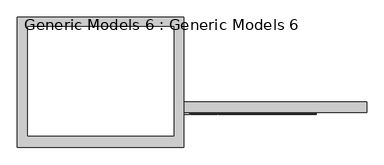
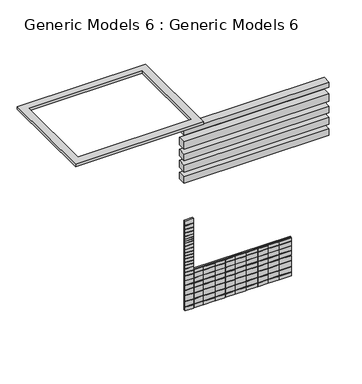
"""IFC4 building model written with IfcOpenShell, lengths in millimetres: proxy geometry, Generic Models 6 : Generic Models 6."""

from ifc_helpers import new_model, si_unit, frame, origin, place, context, project, spatial, polyline, outline, extrude, faceted_brep, source, transform, mapped, element, save


def generic_models_6_generic_models_6_0c77f430(model_context):
    return source(origin(), model_context, "Body", "SolidModel", [
        extrude(outline(polyline([(-18013.9734486, -8229.0592534), (-14420.7831929, -8229.0592534), (-14420.7831929, -11048.4592534), (-18013.9734486, -11048.4592534), (-18013.9734486, -8229.0592534)]), holes=[polyline([(-17794.9964661, -10800.2393368), (-14630.8767684, -10800.2393368), (-14630.8767684, -8432.2592534), (-17794.9964661, -8432.2592534), (-17794.9964661, -10800.2393368)])]), frame((0.0, 0.0, 8571.3431053), z_axis=(0.0, 0.0, 1.0), x_axis=(1.0, 0.0, 0.0)), (0.0, 0.0, 1.0), 76.2),
        extrude(outline(polyline([(-14524.7437117, -10286.4592534), (-14524.7437117, -10057.8592534), (-10464.7331929, -10057.8592534), (-10464.7331929, -10286.4592534), (-14524.7437117, -10286.4592534)])), frame((0.0, 0.0, 6400.8), z_axis=(0.0, 0.0, 1.0), x_axis=(1.0, 0.0, 0.0)), (0.0, 0.0, 1.0), 191.3675565),
        extrude(outline(polyline([(-14524.7437117, -10286.4592534), (-14524.7437117, -10057.8592534), (-10464.7331929, -10057.8592534), (-10464.7331929, -10286.4592534), (-14524.7437117, -10286.4592534)])), frame((0.0, 0.0, 6738.1730597), z_axis=(0.0, 0.0, 1.0), x_axis=(1.0, 0.0, 0.0)), (0.0, 0.0, 1.0), 204.0095282),
        extrude(outline(polyline([(-14524.7437117, -10286.4592534), (-14524.7437117, -10057.8592534), (-10464.7331929, -10057.8592534), (-10464.7331929, -10286.4592534), (-14524.7437117, -10286.4592534)])), frame((0.0, 0.0, 7077.9317925), z_axis=(0.0, 0.0, 1.0), x_axis=(1.0, 0.0, 0.0)), (0.0, 0.0, 1.0), 192.5683417),
        extrude(outline(polyline([(-14524.7437117, -10286.4592534), (-14524.7437117, -10057.8592534), (-10464.7331929, -10057.8592534), (-10464.7331929, -10286.4592534), (-14524.7437117, -10286.4592534)])), frame((0.0, 0.0, 7413.8898365), z_axis=(0.0, 0.0, 1.0), x_axis=(1.0, 0.0, 0.0)), (0.0, 0.0, 1.0), 213.9956527),
        extrude(outline(polyline([(-14524.7437117, -10286.4592534), (-14524.7437117, -10057.8592534), (-10464.7331929, -10057.8592534), (-10464.7331929, -10286.4592534), (-14524.7437117, -10286.4592534)])), frame((0.0, 0.0, 7820.9092835), z_axis=(0.0, 0.0, 1.0), x_axis=(1.0, 0.0, 0.0)), (0.0, 0.0, 1.0), 157.6710883),
        faceted_brep([(-14293.7831929, -10337.2592534, 5313.3697962), (-14524.7437117, -10337.2592534, 5313.3697962), (-14524.7437117, -10337.2592534, 5188.1331788), (-14293.7831929, -10337.2592534, 5188.1331788), (-11550.5831929, -10337.2592534, 3695.8817592), (-11550.5831929, -10337.2592534, 3780.6568837), (-11880.9442119, -10337.2592534, 3780.6568837), (-11880.9442119, -10337.2592534, 3695.8817592), (-11550.5831929, -10337.2592534, 3547.0366558), (-11550.5831929, -10337.2592534, 3680.189393), (-11880.9442119, -10337.2592534, 3680.189393), (-11880.9442119, -10337.2592534, 3547.0366558), (-11550.5831929, -10337.2592534, 3417.1914801), (-11550.5831929, -10337.2592534, 3542.5886948), (-11880.9442119, -10337.2592534, 3542.5886948), (-11880.9442119, -10337.2592534, 3417.1914801), (-11550.5831929, -10337.2592534, 3270.1734591), (-11550.5831929, -10337.2592534, 3393.2583138), (-11880.9442119, -10337.2592534, 3393.2583138), (-11880.9442119, -10337.2592534, 3270.1734591), (-11550.5831929, -10337.2592534, 3111.840506), (-11550.5831929, -10337.2592534, 3253.9449104), (-11880.9442119, -10337.2592534, 3253.9449104), (-11880.9442119, -10337.2592534, 3111.840506), (-11550.5831929, -10337.2592534, 2938.7596873), (-11550.5831929, -10337.2592534, 3096.8139071), (-11880.9442119, -10337.2592534, 3096.8139071), (-11880.9442119, -10337.2592534, 2938.7596873), (-11550.5831929, -10337.2592534, 2659.3923672), (-11550.5831929, -10337.2592534, 2760.4299366), (-11880.9442119, -10337.2592534, 2760.4299366), (-11880.9442119, -10337.2592534, 2659.3923672), (-11550.5831929, -10337.2592534, 2780.6285186), (-11550.5831929, -10337.2592534, 2920.5978973), (-11880.9442119, -10337.2592534, 2920.5978973), (-11880.9442119, -10337.2592534, 2780.6285186), (-14293.7831929, -10337.2592534, 5069.4562317), (-14293.7831929, -10337.2592534, 5168.2265161), (-14524.7437117, -10337.2592534, 5168.2265161), (-14524.7437117, -10337.2592534, 5069.4562317), (-14293.7831929, -10337.2592534, 4965.1249586), (-14293.7831929, -10337.2592534, 5057.6988625), (-14524.7437117, -10337.2592534, 5057.6988625), (-14524.7437117, -10337.2592534, 4965.1249586), (-14293.7831929, -10337.2592534, 4865.3991355), (-14293.7831929, -10337.2592534, 4953.6426938), (-14524.7437117, -10337.2592534, 4953.6426938), (-14524.7437117, -10337.2592534, 4865.3991355), (-14293.7831929, -10337.2592534, 4781.0487347), (-14293.7831929, -10337.2592534, 4856.4332696), (-14524.7437117, -10337.2592534, 4856.4332696), (-14524.7437117, -10337.2592534, 4781.0487347), (-14293.7831929, -10337.2592534, 4721.3683685), (-14293.7831929, -10337.2592534, 4774.4107583), (-14524.7437117, -10337.2592534, 4774.4107583), (-14524.7437117, -10337.2592534, 4721.3683685), (-14293.7831929, -10337.2592534, 4665.5616831), (-14293.7831929, -10337.2592534, 4715.3945526), (-14524.7437117, -10337.2592534, 4715.3945526), (-14524.7437117, -10337.2592534, 4665.5616831), (-14293.7831929, -10337.2592534, 4571.464179), (-14293.7831929, -10337.2592534, 4658.9302933), (-14524.7437117, -10337.2592534, 4658.9302933), (-14524.7437117, -10337.2592534, 4571.464179), (-14293.7831929, -10337.2592534, 4470.4894096), (-14293.7831929, -10337.2592534, 4556.4765983), (-14524.7437117, -10337.2592534, 4556.4765983), (-14524.7437117, -10337.2592534, 4470.4894096), (-14293.7831929, -10337.2592534, 4373.4391753), (-14293.7831929, -10337.2592534, 4459.0931873), (-14524.7437117, -10337.2592534, 4459.0931873), (-14524.7437117, -10337.2592534, 4373.4391753), (-14293.7831929, -10337.2592534, 4282.1802011), (-14293.7831929, -10337.2592534, 4359.300461), (-14524.7437117, -10337.2592534, 4359.300461), (-14524.7437117, -10337.2592534, 4282.1802011), (-14293.7831929, -10337.2592534, 4193.4919021), (-14293.7831929, -10337.2592534, 4269.3268244), (-14524.7437117, -10337.2592534, 4269.3268244), (-14524.7437117, -10337.2592534, 4193.4919021), (-14293.7831929, -10337.2592534, 4094.064607), (-14293.7831929, -10337.2592534, 4178.0678501), (-14524.7437117, -10337.2592534, 4178.0678501), (-14524.7437117, -10337.2592534, 4094.064607), (-14293.7831929, -10337.2592534, 4000.5723585), (-14293.7831929, -10337.2592534, 4078.7658754), (-14524.7437117, -10337.2592534, 4078.7658754), (-14524.7437117, -10337.2592534, 4000.5723585), (-14293.7831929, -10337.2592534, 3799.5834003), (-14293.7831929, -10337.2592534, 3891.5162081), (-14524.7437117, -10337.2592534, 3891.5162081), (-14524.7437117, -10337.2592534, 3799.5834003), (-14293.7831929, -10337.2592534, 3900.2806738), (-14293.7831929, -10337.2592534, 3986.3810817), (-14524.7437117, -10337.2592534, 3986.3810817), (-14524.7437117, -10337.2592534, 3900.2806738), (-14524.7437117, -10337.2592534, 3780.6568837), (-14524.7437117, -10337.2592534, 3695.8817592), (-14293.7831929, -10337.2592534, 3695.8817592), (-14293.7831929, -10337.2592534, 3780.6568837), (-14524.7437117, -10337.2592534, 3680.189393), (-14524.7437117, -10337.2592534, 3547.0366558), (-14293.7831929, -10337.2592534, 3547.0366558), (-14293.7831929, -10337.2592534, 3680.189393), (-14524.7437117, -10337.2592534, 3542.5886948), (-14524.7437117, -10337.2592534, 3417.1914801), (-14293.7831929, -10337.2592534, 3417.1914801), (-14293.7831929, -10337.2592534, 3542.5886948), (-14524.7437117, -10337.2592534, 3393.2583138), (-14524.7437117, -10337.2592534, 3270.1734591), (-14293.7831929, -10337.2592534, 3270.1734591), (-14293.7831929, -10337.2592534, 3393.2583138), (-14524.7437117, -10337.2592534, 3253.9449104), (-14524.7437117, -10337.2592534, 3111.840506), (-14293.7831929, -10337.2592534, 3111.840506), (-14293.7831929, -10337.2592534, 3253.9449104), (-14524.7437117, -10337.2592534, 3096.8139071), (-14524.7437117, -10337.2592534, 2938.7596873), (-14293.7831929, -10337.2592534, 2938.7596873), (-14293.7831929, -10337.2592534, 3096.8139071), (-14524.7437117, -10337.2592534, 2760.4299366), (-14524.7437117, -10337.2592534, 2659.3923672), (-14293.7831929, -10337.2592534, 2659.3923672), (-14293.7831929, -10337.2592534, 2760.4299366), (-14524.7437117, -10337.2592534, 2920.5978973), (-14524.7437117, -10337.2592534, 2780.6285186), (-14293.7831929, -10337.2592534, 2780.6285186), (-14293.7831929, -10337.2592534, 2920.5978973), (-14277.8960614, -10337.2592534, 2659.3923672), (-14019.6359859, -10337.2592534, 2659.3923672), (-14019.6359859, -10337.2592534, 2760.4299366), (-14277.8960614, -10337.2592534, 2760.4299366), (-14004.4843067, -10337.2592534, 2659.3923672), (-13695.1641924, -10337.2592534, 2659.3923672), (-13695.1641924, -10337.2592534, 2760.4299366), (-14004.4843067, -10337.2592534, 2760.4299366), (-13674.725498, -10337.2592534, 2659.3923672), (-13411.1331929, -10337.2592534, 2659.3923672), (-13411.1331929, -10337.2592534, 2760.4299366), (-13674.725498, -10337.2592534, 2760.4299366), (-13398.4331929, -10337.2592534, 2659.3923672), (-13132.6036786, -10337.2592534, 2659.3923672), (-13132.6036786, -10337.2592534, 2760.4299366), (-13398.4331929, -10337.2592534, 2760.4299366), (-13122.8488627, -10337.2592534, 2659.3923672), (-12816.2756326, -10337.2592534, 2659.3923672), (-12816.2756326, -10337.2592534, 2760.4299366), (-13122.8488627, -10337.2592534, 2760.4299366), (-12805.7258669, -10337.2592534, 2659.3923672), (-12496.7331929, -10337.2592534, 2659.3923672), (-12496.7331929, -10337.2592534, 2760.4299366), (-12805.7258669, -10337.2592534, 2760.4299366), (-12491.0846074, -10337.2592534, 2659.3923672), (-12209.2160936, -10337.2592534, 2659.3923672), (-12209.2160936, -10337.2592534, 2760.4299366), (-12491.0846074, -10337.2592534, 2760.4299366), (-12202.6421379, -10337.2592534, 2659.3923672), (-11888.3927856, -10337.2592534, 2659.3923672), (-11888.3927856, -10337.2592534, 2760.4299366), (-12202.6421379, -10337.2592534, 2760.4299366), (-14019.6359859, -10337.2592534, 3780.6568837), (-14277.8960614, -10337.2592534, 3780.6568837), (-14277.8960614, -10337.2592534, 3695.8817592), (-14019.6359859, -10337.2592534, 3695.8817592), (-13695.1641924, -10337.2592534, 3780.6568837), (-14004.4843067, -10337.2592534, 3780.6568837), (-14004.4843067, -10337.2592534, 3695.8817592), (-13695.1641924, -10337.2592534, 3695.8817592), (-13411.1331929, -10337.2592534, 3780.6568837), (-13674.725498, -10337.2592534, 3780.6568837), (-13674.725498, -10337.2592534, 3695.8817592), (-13411.1331929, -10337.2592534, 3695.8817592), (-13132.6036786, -10337.2592534, 3780.6568837), (-13398.4331929, -10337.2592534, 3780.6568837), (-13398.4331929, -10337.2592534, 3695.8817592), (-13132.6036786, -10337.2592534, 3695.8817592), (-12816.2756326, -10337.2592534, 3780.6568837), (-13122.8488627, -10337.2592534, 3780.6568837), (-13122.8488627, -10337.2592534, 3695.8817592), (-12816.2756326, -10337.2592534, 3695.8817592), (-12496.7331929, -10337.2592534, 3780.6568837), (-12805.7258669, -10337.2592534, 3780.6568837), (-12805.7258669, -10337.2592534, 3695.8817592), (-12496.7331929, -10337.2592534, 3695.8817592), (-12209.2160936, -10337.2592534, 3780.6568837), (-12491.0846074, -10337.2592534, 3780.6568837), (-12491.0846074, -10337.2592534, 3695.8817592), (-12209.2160936, -10337.2592534, 3695.8817592), (-11888.3927856, -10337.2592534, 3780.6568837), (-12202.6421379, -10337.2592534, 3780.6568837), (-12202.6421379, -10337.2592534, 3695.8817592), (-11888.3927856, -10337.2592534, 3695.8817592), (-14019.6359859, -10337.2592534, 3680.189393), (-14277.8960614, -10337.2592534, 3680.189393), (-14277.8960614, -10337.2592534, 3547.0366558), (-14019.6359859, -10337.2592534, 3547.0366558), (-13695.1641924, -10337.2592534, 3680.189393), (-14004.4843067, -10337.2592534, 3680.189393), (-14004.4843067, -10337.2592534, 3547.0366558), (-13695.1641924, -10337.2592534, 3547.0366558), (-13411.1331929, -10337.2592534, 3680.189393), (-13674.725498, -10337.2592534, 3680.189393), (-13674.725498, -10337.2592534, 3547.0366558), (-13411.1331929, -10337.2592534, 3547.0366558), (-13132.6036786, -10337.2592534, 3680.189393), (-13398.4331929, -10337.2592534, 3680.189393), (-13398.4331929, -10337.2592534, 3547.0366558), (-13132.6036786, -10337.2592534, 3547.0366558), (-12816.2756326, -10337.2592534, 3680.189393), (-13122.8488627, -10337.2592534, 3680.189393), (-13122.8488627, -10337.2592534, 3547.0366558), (-12816.2756326, -10337.2592534, 3547.0366558), (-12496.7331929, -10337.2592534, 3680.189393), (-12805.7258669, -10337.2592534, 3680.189393), (-12805.7258669, -10337.2592534, 3547.0366558), (-12496.7331929, -10337.2592534, 3547.0366558), (-12209.2160936, -10337.2592534, 3680.189393), (-12491.0846074, -10337.2592534, 3680.189393), (-12491.0846074, -10337.2592534, 3547.0366558), (-12209.2160936, -10337.2592534, 3547.0366558), (-11888.3927856, -10337.2592534, 3680.189393), (-12202.6421379, -10337.2592534, 3680.189393), (-12202.6421379, -10337.2592534, 3547.0366558), (-11888.3927856, -10337.2592534, 3547.0366558), (-14019.6359859, -10337.2592534, 3542.5886948), (-14277.8960614, -10337.2592534, 3542.5886948), (-14277.8960614, -10337.2592534, 3417.1914801), (-14019.6359859, -10337.2592534, 3417.1914801), (-13695.1641924, -10337.2592534, 3542.5886948), (-14004.4843067, -10337.2592534, 3542.5886948), (-14004.4843067, -10337.2592534, 3417.1914801), (-13695.1641924, -10337.2592534, 3417.1914801), (-13411.1331929, -10337.2592534, 3542.5886948), (-13674.725498, -10337.2592534, 3542.5886948), (-13674.725498, -10337.2592534, 3417.1914801), (-13411.1331929, -10337.2592534, 3417.1914801), (-13132.6036786, -10337.2592534, 3542.5886948), (-13398.4331929, -10337.2592534, 3542.5886948), (-13398.4331929, -10337.2592534, 3417.1914801), (-13132.6036786, -10337.2592534, 3417.1914801), (-12816.2756326, -10337.2592534, 3542.5886948), (-13122.8488627, -10337.2592534, 3542.5886948), (-13122.8488627, -10337.2592534, 3417.1914801), (-12816.2756326, -10337.2592534, 3417.1914801), (-12496.7331929, -10337.2592534, 3542.5886948), (-12805.7258669, -10337.2592534, 3542.5886948), (-12805.7258669, -10337.2592534, 3417.1914801), (-12496.7331929, -10337.2592534, 3417.1914801), (-12209.2160936, -10337.2592534, 3542.5886948), (-12491.0846074, -10337.2592534, 3542.5886948), (-12491.0846074, -10337.2592534, 3417.1914801), (-12209.2160936, -10337.2592534, 3417.1914801), (-11888.3927856, -10337.2592534, 3542.5886948), (-12202.6421379, -10337.2592534, 3542.5886948), (-12202.6421379, -10337.2592534, 3417.1914801), (-11888.3927856, -10337.2592534, 3417.1914801), (-14019.6359859, -10337.2592534, 3393.2583138), (-14277.8960614, -10337.2592534, 3393.2583138), (-14277.8960614, -10337.2592534, 3270.1734591), (-14019.6359859, -10337.2592534, 3270.1734591), (-13695.1641924, -10337.2592534, 3393.2583138), (-14004.4843067, -10337.2592534, 3393.2583138), (-14004.4843067, -10337.2592534, 3270.1734591), (-13695.1641924, -10337.2592534, 3270.1734591), (-13411.1331929, -10337.2592534, 3393.2583138), (-13674.725498, -10337.2592534, 3393.2583138), (-13674.725498, -10337.2592534, 3270.1734591), (-13411.1331929, -10337.2592534, 3270.1734591), (-13132.6036786, -10337.2592534, 3393.2583138), (-13398.4331929, -10337.2592534, 3393.2583138), (-13398.4331929, -10337.2592534, 3270.1734591), (-13132.6036786, -10337.2592534, 3270.1734591), (-12816.2756326, -10337.2592534, 3393.2583138), (-13122.8488627, -10337.2592534, 3393.2583138), (-13122.8488627, -10337.2592534, 3270.1734591), (-12816.2756326, -10337.2592534, 3270.1734591), (-12496.7331929, -10337.2592534, 3393.2583138), (-12805.7258669, -10337.2592534, 3393.2583138), (-12805.7258669, -10337.2592534, 3270.1734591), (-12496.7331929, -10337.2592534, 3270.1734591), (-12209.2160936, -10337.2592534, 3393.2583138), (-12491.0846074, -10337.2592534, 3393.2583138), (-12491.0846074, -10337.2592534, 3270.1734591), (-12209.2160936, -10337.2592534, 3270.1734591), (-11888.3927856, -10337.2592534, 3393.2583138), (-12202.6421379, -10337.2592534, 3393.2583138), (-12202.6421379, -10337.2592534, 3270.1734591), (-11888.3927856, -10337.2592534, 3270.1734591), (-14019.6359859, -10337.2592534, 3253.9449104), (-14277.8960614, -10337.2592534, 3253.9449104), (-14277.8960614, -10337.2592534, 3111.840506), (-14019.6359859, -10337.2592534, 3111.840506), (-13695.1641924, -10337.2592534, 3253.9449104), (-14004.4843067, -10337.2592534, 3253.9449104), (-14004.4843067, -10337.2592534, 3111.840506), (-13695.1641924, -10337.2592534, 3111.840506), (-13411.1331929, -10337.2592534, 3253.9449104), (-13674.725498, -10337.2592534, 3253.9449104), (-13674.725498, -10337.2592534, 3111.840506), (-13411.1331929, -10337.2592534, 3111.840506), (-13132.6036786, -10337.2592534, 3253.9449104), (-13398.4331929, -10337.2592534, 3253.9449104), (-13398.4331929, -10337.2592534, 3111.840506), (-13132.6036786, -10337.2592534, 3111.840506), (-12816.2756326, -10337.2592534, 3253.9449104), (-13122.8488627, -10337.2592534, 3253.9449104), (-13122.8488627, -10337.2592534, 3111.840506), (-12816.2756326, -10337.2592534, 3111.840506), (-12496.7331929, -10337.2592534, 3253.9449104), (-12805.7258669, -10337.2592534, 3253.9449104), (-12805.7258669, -10337.2592534, 3111.840506), (-12496.7331929, -10337.2592534, 3111.840506), (-12209.2160936, -10337.2592534, 3253.9449104), (-12491.0846074, -10337.2592534, 3253.9449104), (-12491.0846074, -10337.2592534, 3111.840506), (-12209.2160936, -10337.2592534, 3111.840506), (-11888.3927856, -10337.2592534, 3253.9449104), (-12202.6421379, -10337.2592534, 3253.9449104), (-12202.6421379, -10337.2592534, 3111.840506), (-11888.3927856, -10337.2592534, 3111.840506), (-14019.6359859, -10337.2592534, 3096.8139071), (-14277.8960614, -10337.2592534, 3096.8139071), (-14277.8960614, -10337.2592534, 2938.7596873), (-14019.6359859, -10337.2592534, 2938.7596873), (-13695.1641924, -10337.2592534, 3096.8139071), (-14004.4843067, -10337.2592534, 3096.8139071), (-14004.4843067, -10337.2592534, 2938.7596873), (-13695.1641924, -10337.2592534, 2938.7596873), (-13411.1331929, -10337.2592534, 3096.8139071), (-13674.725498, -10337.2592534, 3096.8139071), (-13674.725498, -10337.2592534, 2938.7596873), (-13411.1331929, -10337.2592534, 2938.7596873), (-13132.6036786, -10337.2592534, 3096.8139071), (-13398.4331929, -10337.2592534, 3096.8139071), (-13398.4331929, -10337.2592534, 2938.7596873), (-13132.6036786, -10337.2592534, 2938.7596873), (-12816.2756326, -10337.2592534, 3096.8139071), (-13122.8488627, -10337.2592534, 3096.8139071), (-13122.8488627, -10337.2592534, 2938.7596873), (-12816.2756326, -10337.2592534, 2938.7596873), (-12496.7331929, -10337.2592534, 3096.8139071), (-12805.7258669, -10337.2592534, 3096.8139071), (-12805.7258669, -10337.2592534, 2938.7596873), (-12496.7331929, -10337.2592534, 2938.7596873), (-12209.2160936, -10337.2592534, 3096.8139071), (-12491.0846074, -10337.2592534, 3096.8139071), (-12491.0846074, -10337.2592534, 2938.7596873), (-12209.2160936, -10337.2592534, 2938.7596873), (-11888.3927856, -10337.2592534, 3096.8139071), (-12202.6421379, -10337.2592534, 3096.8139071), (-12202.6421379, -10337.2592534, 2938.7596873), (-11888.3927856, -10337.2592534, 2938.7596873), (-14019.6359859, -10337.2592534, 2920.5978973), (-14277.8960614, -10337.2592534, 2920.5978973), (-14277.8960614, -10337.2592534, 2780.6285186), (-14019.6359859, -10337.2592534, 2780.6285186), (-13695.1641924, -10337.2592534, 2920.5978973), (-14004.4843067, -10337.2592534, 2920.5978973), (-14004.4843067, -10337.2592534, 2780.6285186), (-13695.1641924, -10337.2592534, 2780.6285186), (-13411.1331929, -10337.2592534, 2920.5978973), (-13674.725498, -10337.2592534, 2920.5978973), (-13674.725498, -10337.2592534, 2780.6285186), (-13411.1331929, -10337.2592534, 2780.6285186), (-13132.6036786, -10337.2592534, 2920.5978973), (-13398.4331929, -10337.2592534, 2920.5978973), (-13398.4331929, -10337.2592534, 2780.6285186), (-13132.6036786, -10337.2592534, 2780.6285186), (-12816.2756326, -10337.2592534, 2920.5978973), (-13122.8488627, -10337.2592534, 2920.5978973), (-13122.8488627, -10337.2592534, 2780.6285186), (-12816.2756326, -10337.2592534, 2780.6285186), (-12496.7331929, -10337.2592534, 2920.5978973), (-12805.7258669, -10337.2592534, 2920.5978973), (-12805.7258669, -10337.2592534, 2780.6285186), (-12496.7331929, -10337.2592534, 2780.6285186), (-12209.2160936, -10337.2592534, 2920.5978973), (-12491.0846074, -10337.2592534, 2920.5978973), (-12491.0846074, -10337.2592534, 2780.6285186), (-12209.2160936, -10337.2592534, 2780.6285186), (-11888.3927856, -10337.2592534, 2920.5978973), (-12202.6421379, -10337.2592534, 2920.5978973), (-12202.6421379, -10337.2592534, 2780.6285186), (-11888.3927856, -10337.2592534, 2780.6285186), (-11550.5831929, -10286.4592534, 3799.5834003), (-11550.5831929, -10286.4592534, 2659.3923672), (-14524.7437117, -10286.4592534, 2659.3923672), (-14524.7437117, -10286.4592534, 5313.3697962), (-14293.7831929, -10286.4592534, 5313.3697962), (-14293.7831929, -10286.4592534, 3799.5834003), (-14293.7831929, -10311.8592534, 3799.5834003), (-11550.5831929, -10311.8592534, 3799.5834003), (-14524.7437117, -10311.8592534, 2760.4299366), (-14524.7437117, -10311.8592534, 2780.6285186), (-14524.7437117, -10311.8592534, 2920.5978973), (-14524.7437117, -10311.8592534, 2938.7596873), (-14524.7437117, -10311.8592534, 3096.8139071), (-14524.7437117, -10311.8592534, 3111.840506), (-14524.7437117, -10311.8592534, 3253.9449104), (-14524.7437117, -10311.8592534, 3270.1734591), (-14524.7437117, -10311.8592534, 3393.2583138), (-14524.7437117, -10311.8592534, 3417.1914801), (-14524.7437117, -10311.8592534, 3542.5886948), (-14524.7437117, -10311.8592534, 3547.0366558), (-14524.7437117, -10311.8592534, 3680.189393), (-14524.7437117, -10311.8592534, 3695.8817592), (-14524.7437117, -10311.8592534, 3780.6568837), (-14524.7437117, -10311.8592534, 3799.5834003), (-14524.7437117, -10311.8592534, 3891.5162081), (-14524.7437117, -10311.8592534, 3900.2806738), (-14524.7437117, -10311.8592534, 3986.3810817), (-14524.7437117, -10311.8592534, 4000.5723585), (-14524.7437117, -10311.8592534, 4078.7658754), (-14524.7437117, -10311.8592534, 4094.064607), (-14524.7437117, -10311.8592534, 4178.0678501), (-14524.7437117, -10311.8592534, 4193.4919021), (-14524.7437117, -10311.8592534, 4269.3268244), (-14524.7437117, -10311.8592534, 4282.1802011), (-14524.7437117, -10311.8592534, 4359.300461), (-14524.7437117, -10311.8592534, 4373.4391753), (-14524.7437117, -10311.8592534, 4459.0931873), (-14524.7437117, -10311.8592534, 4470.4894096), (-14524.7437117, -10311.8592534, 4556.4765983), (-14524.7437117, -10311.8592534, 4571.464179), (-14524.7437117, -10311.8592534, 4658.9302933), (-14524.7437117, -10311.8592534, 4665.5616831), (-14524.7437117, -10311.8592534, 4715.3945526), (-14524.7437117, -10311.8592534, 4721.3683685), (-14524.7437117, -10311.8592534, 4774.4107583), (-14524.7437117, -10311.8592534, 4781.0487347), (-14524.7437117, -10311.8592534, 4856.4332696), (-14524.7437117, -10311.8592534, 4865.3991355), (-14524.7437117, -10311.8592534, 4953.6426938), (-14524.7437117, -10311.8592534, 4965.1249586), (-14524.7437117, -10311.8592534, 5057.6988625), (-14524.7437117, -10311.8592534, 5069.4562317), (-14524.7437117, -10311.8592534, 5168.2265161), (-14524.7437117, -10311.8592534, 5188.1331788), (-11880.9442119, -10311.8592534, 2659.3923672), (-11888.3927856, -10311.8592534, 2659.3923672), (-12202.6421379, -10311.8592534, 2659.3923672), (-12209.2160936, -10311.8592534, 2659.3923672), (-12491.0846074, -10311.8592534, 2659.3923672), (-12496.7331929, -10311.8592534, 2659.3923672), (-12805.7258669, -10311.8592534, 2659.3923672), (-12816.2756326, -10311.8592534, 2659.3923672), (-13122.8488627, -10311.8592534, 2659.3923672), (-13132.6036786, -10311.8592534, 2659.3923672), (-13398.4331929, -10311.8592534, 2659.3923672), (-13411.1331929, -10311.8592534, 2659.3923672), (-13674.725498, -10311.8592534, 2659.3923672), (-13695.1641924, -10311.8592534, 2659.3923672), (-14004.4843067, -10311.8592534, 2659.3923672), (-14019.6359859, -10311.8592534, 2659.3923672), (-14277.8960614, -10311.8592534, 2659.3923672), (-14293.7831929, -10311.8592534, 2659.3923672), (-11550.5831929, -10311.8592534, 3780.6568837), (-11550.5831929, -10311.8592534, 3695.8817592), (-11550.5831929, -10311.8592534, 3680.189393), (-11550.5831929, -10311.8592534, 3547.0366558), (-11550.5831929, -10311.8592534, 3542.5886948), (-11550.5831929, -10311.8592534, 3417.1914801), (-11550.5831929, -10311.8592534, 3393.2583138), (-11550.5831929, -10311.8592534, 3270.1734591), (-11550.5831929, -10311.8592534, 3253.9449104), (-11550.5831929, -10311.8592534, 3111.840506), (-11550.5831929, -10311.8592534, 3096.8139071), (-11550.5831929, -10311.8592534, 2938.7596873), (-11550.5831929, -10311.8592534, 2920.5978973), (-11550.5831929, -10311.8592534, 2780.6285186), (-11550.5831929, -10311.8592534, 2760.4299366), (-14293.7831929, -10311.8592534, 5188.1331788), (-14293.7831929, -10311.8592534, 5168.2265161), (-14293.7831929, -10311.8592534, 5069.4562317), (-14293.7831929, -10311.8592534, 5057.6988625), (-14293.7831929, -10311.8592534, 4965.1249586), (-14293.7831929, -10311.8592534, 4953.6426938), (-14293.7831929, -10311.8592534, 4865.3991355), (-14293.7831929, -10311.8592534, 4856.4332696), (-14293.7831929, -10311.8592534, 4781.0487347), (-14293.7831929, -10311.8592534, 4774.4107583), (-14293.7831929, -10311.8592534, 4721.3683685), (-14293.7831929, -10311.8592534, 4715.3945526), (-14293.7831929, -10311.8592534, 4665.5616831), (-14293.7831929, -10311.8592534, 4658.9302933), (-14293.7831929, -10311.8592534, 4571.464179), (-14293.7831929, -10311.8592534, 4556.4765983), (-14293.7831929, -10311.8592534, 4470.4894096), (-14293.7831929, -10311.8592534, 4459.0931873), (-14293.7831929, -10311.8592534, 4373.4391753), (-14293.7831929, -10311.8592534, 4359.300461), (-14293.7831929, -10311.8592534, 4282.1802011), (-14293.7831929, -10311.8592534, 4269.3268244), (-14293.7831929, -10311.8592534, 4193.4919021), (-14293.7831929, -10311.8592534, 4178.0678501), (-14293.7831929, -10311.8592534, 4094.064607), (-14293.7831929, -10311.8592534, 4078.7658754), (-14293.7831929, -10311.8592534, 4000.5723585), (-14293.7831929, -10311.8592534, 3986.3810817), (-14293.7831929, -10311.8592534, 3900.2806738), (-14293.7831929, -10311.8592534, 3891.5162081), (-14293.7831929, -10311.8592534, 3780.6568837), (-14293.7831929, -10311.8592534, 3695.8817592), (-14293.7831929, -10311.8592534, 3680.189393), (-14293.7831929, -10311.8592534, 3547.0366558), (-14293.7831929, -10311.8592534, 3542.5886948), (-14293.7831929, -10311.8592534, 3417.1914801), (-14293.7831929, -10311.8592534, 3393.2583138), (-14293.7831929, -10311.8592534, 3270.1734591), (-14293.7831929, -10311.8592534, 3253.9449104), (-14293.7831929, -10311.8592534, 3111.840506), (-14293.7831929, -10311.8592534, 3096.8139071), (-14293.7831929, -10311.8592534, 2938.7596873), (-14293.7831929, -10311.8592534, 2920.5978973), (-14293.7831929, -10311.8592534, 2780.6285186), (-14293.7831929, -10311.8592534, 2760.4299366), (-14277.8960614, -10311.8592534, 2760.4299366), (-14019.6359859, -10311.8592534, 2760.4299366), (-14004.4843067, -10311.8592534, 2760.4299366), (-13695.1641924, -10311.8592534, 2760.4299366), (-13674.725498, -10311.8592534, 2760.4299366), (-13411.1331929, -10311.8592534, 2760.4299366), (-13398.4331929, -10311.8592534, 2760.4299366), (-13132.6036786, -10311.8592534, 2760.4299366), (-13122.8488627, -10311.8592534, 2760.4299366), (-12816.2756326, -10311.8592534, 2760.4299366), (-12805.7258669, -10311.8592534, 2760.4299366), (-12496.7331929, -10311.8592534, 2760.4299366), (-12491.0846074, -10311.8592534, 2760.4299366), (-12209.2160936, -10311.8592534, 2760.4299366), (-12202.6421379, -10311.8592534, 2760.4299366), (-11888.3927856, -10311.8592534, 2760.4299366), (-11880.9442119, -10311.8592534, 2760.4299366), (-11880.9442119, -10311.8592534, 2780.6285186), (-11880.9442119, -10311.8592534, 2920.5978973), (-11880.9442119, -10311.8592534, 2938.7596873), (-11880.9442119, -10311.8592534, 3096.8139071), (-11880.9442119, -10311.8592534, 3111.840506), (-11880.9442119, -10311.8592534, 3253.9449104), (-11880.9442119, -10311.8592534, 3270.1734591), (-11880.9442119, -10311.8592534, 3393.2583138), (-11880.9442119, -10311.8592534, 3417.1914801), (-11880.9442119, -10311.8592534, 3542.5886948), (-11880.9442119, -10311.8592534, 3547.0366558), (-11880.9442119, -10311.8592534, 3680.189393), (-11880.9442119, -10311.8592534, 3695.8817592), (-11880.9442119, -10311.8592534, 3780.6568837), (-14277.8960614, -10311.8592534, 3780.6568837), (-14019.6359859, -10311.8592534, 3780.6568837), (-14019.6359859, -10311.8592534, 3695.8817592), (-14277.8960614, -10311.8592534, 3695.8817592), (-14004.4843067, -10311.8592534, 3780.6568837), (-13695.1641924, -10311.8592534, 3780.6568837), (-13695.1641924, -10311.8592534, 3695.8817592), (-14004.4843067, -10311.8592534, 3695.8817592), (-13674.725498, -10311.8592534, 3780.6568837), (-13411.1331929, -10311.8592534, 3780.6568837), (-13411.1331929, -10311.8592534, 3695.8817592), (-13674.725498, -10311.8592534, 3695.8817592), (-13398.4331929, -10311.8592534, 3780.6568837), (-13132.6036786, -10311.8592534, 3780.6568837), (-13132.6036786, -10311.8592534, 3695.8817592), (-13398.4331929, -10311.8592534, 3695.8817592), (-13122.8488627, -10311.8592534, 3780.6568837), (-12816.2756326, -10311.8592534, 3780.6568837), (-12816.2756326, -10311.8592534, 3695.8817592), (-13122.8488627, -10311.8592534, 3695.8817592), (-12805.7258669, -10311.8592534, 3780.6568837), (-12496.7331929, -10311.8592534, 3780.6568837), (-12496.7331929, -10311.8592534, 3695.8817592), (-12805.7258669, -10311.8592534, 3695.8817592), (-12491.0846074, -10311.8592534, 3780.6568837), (-12209.2160936, -10311.8592534, 3780.6568837), (-12209.2160936, -10311.8592534, 3695.8817592), (-12491.0846074, -10311.8592534, 3695.8817592), (-12202.6421379, -10311.8592534, 3780.6568837), (-11888.3927856, -10311.8592534, 3780.6568837), (-11888.3927856, -10311.8592534, 3695.8817592), (-12202.6421379, -10311.8592534, 3695.8817592), (-14277.8960614, -10311.8592534, 3680.189393), (-14019.6359859, -10311.8592534, 3680.189393), (-14019.6359859, -10311.8592534, 3547.0366558), (-14277.8960614, -10311.8592534, 3547.0366558), (-14004.4843067, -10311.8592534, 3680.189393), (-13695.1641924, -10311.8592534, 3680.189393), (-13695.1641924, -10311.8592534, 3547.0366558), (-14004.4843067, -10311.8592534, 3547.0366558), (-13674.725498, -10311.8592534, 3680.189393), (-13411.1331929, -10311.8592534, 3680.189393), (-13411.1331929, -10311.8592534, 3547.0366558), (-13674.725498, -10311.8592534, 3547.0366558), (-13398.4331929, -10311.8592534, 3680.189393), (-13132.6036786, -10311.8592534, 3680.189393), (-13132.6036786, -10311.8592534, 3547.0366558), (-13398.4331929, -10311.8592534, 3547.0366558), (-13122.8488627, -10311.8592534, 3680.189393), (-12816.2756326, -10311.8592534, 3680.189393), (-12816.2756326, -10311.8592534, 3547.0366558), (-13122.8488627, -10311.8592534, 3547.0366558), (-12805.7258669, -10311.8592534, 3680.189393), (-12496.7331929, -10311.8592534, 3680.189393), (-12496.7331929, -10311.8592534, 3547.0366558), (-12805.7258669, -10311.8592534, 3547.0366558), (-12491.0846074, -10311.8592534, 3680.189393), (-12209.2160936, -10311.8592534, 3680.189393), (-12209.2160936, -10311.8592534, 3547.0366558), (-12491.0846074, -10311.8592534, 3547.0366558), (-12202.6421379, -10311.8592534, 3680.189393), (-11888.3927856, -10311.8592534, 3680.189393), (-11888.3927856, -10311.8592534, 3547.0366558), (-12202.6421379, -10311.8592534, 3547.0366558), (-14277.8960614, -10311.8592534, 3542.5886948), (-14019.6359859, -10311.8592534, 3542.5886948), (-14019.6359859, -10311.8592534, 3417.1914801), (-14277.8960614, -10311.8592534, 3417.1914801), (-14004.4843067, -10311.8592534, 3542.5886948), (-13695.1641924, -10311.8592534, 3542.5886948), (-13695.1641924, -10311.8592534, 3417.1914801), (-14004.4843067, -10311.8592534, 3417.1914801), (-13674.725498, -10311.8592534, 3542.5886948), (-13411.1331929, -10311.8592534, 3542.5886948), (-13411.1331929, -10311.8592534, 3417.1914801), (-13674.725498, -10311.8592534, 3417.1914801), (-13398.4331929, -10311.8592534, 3542.5886948), (-13132.6036786, -10311.8592534, 3542.5886948), (-13132.6036786, -10311.8592534, 3417.1914801), (-13398.4331929, -10311.8592534, 3417.1914801), (-13122.8488627, -10311.8592534, 3542.5886948), (-12816.2756326, -10311.8592534, 3542.5886948), (-12816.2756326, -10311.8592534, 3417.1914801), (-13122.8488627, -10311.8592534, 3417.1914801), (-12805.7258669, -10311.8592534, 3542.5886948), (-12496.7331929, -10311.8592534, 3542.5886948), (-12496.7331929, -10311.8592534, 3417.1914801), (-12805.7258669, -10311.8592534, 3417.1914801), (-12491.0846074, -10311.8592534, 3542.5886948), (-12209.2160936, -10311.8592534, 3542.5886948), (-12209.2160936, -10311.8592534, 3417.1914801), (-12491.0846074, -10311.8592534, 3417.1914801), (-12202.6421379, -10311.8592534, 3542.5886948), (-11888.3927856, -10311.8592534, 3542.5886948), (-11888.3927856, -10311.8592534, 3417.1914801), (-12202.6421379, -10311.8592534, 3417.1914801), (-14277.8960614, -10311.8592534, 3393.2583138), (-14019.6359859, -10311.8592534, 3393.2583138), (-14019.6359859, -10311.8592534, 3270.1734591), (-14277.8960614, -10311.8592534, 3270.1734591), (-14004.4843067, -10311.8592534, 3393.2583138), (-13695.1641924, -10311.8592534, 3393.2583138), (-13695.1641924, -10311.8592534, 3270.1734591), (-14004.4843067, -10311.8592534, 3270.1734591), (-13674.725498, -10311.8592534, 3393.2583138), (-13411.1331929, -10311.8592534, 3393.2583138), (-13411.1331929, -10311.8592534, 3270.1734591), (-13674.725498, -10311.8592534, 3270.1734591), (-13398.4331929, -10311.8592534, 3393.2583138), (-13132.6036786, -10311.8592534, 3393.2583138), (-13132.6036786, -10311.8592534, 3270.1734591), (-13398.4331929, -10311.8592534, 3270.1734591), (-13122.8488627, -10311.8592534, 3393.2583138), (-12816.2756326, -10311.8592534, 3393.2583138), (-12816.2756326, -10311.8592534, 3270.1734591), (-13122.8488627, -10311.8592534, 3270.1734591), (-12805.7258669, -10311.8592534, 3393.2583138), (-12496.7331929, -10311.8592534, 3393.2583138), (-12496.7331929, -10311.8592534, 3270.1734591), (-12805.7258669, -10311.8592534, 3270.1734591), (-12491.0846074, -10311.8592534, 3393.2583138), (-12209.2160936, -10311.8592534, 3393.2583138), (-12209.2160936, -10311.8592534, 3270.1734591), (-12491.0846074, -10311.8592534, 3270.1734591), (-12202.6421379, -10311.8592534, 3393.2583138), (-11888.3927856, -10311.8592534, 3393.2583138), (-11888.3927856, -10311.8592534, 3270.1734591), (-12202.6421379, -10311.8592534, 3270.1734591), (-14277.8960614, -10311.8592534, 3253.9449104), (-14019.6359859, -10311.8592534, 3253.9449104), (-14019.6359859, -10311.8592534, 3111.840506), (-14277.8960614, -10311.8592534, 3111.840506), (-14004.4843067, -10311.8592534, 3253.9449104), (-13695.1641924, -10311.8592534, 3253.9449104), (-13695.1641924, -10311.8592534, 3111.840506), (-14004.4843067, -10311.8592534, 3111.840506), (-13674.725498, -10311.8592534, 3253.9449104), (-13411.1331929, -10311.8592534, 3253.9449104), (-13411.1331929, -10311.8592534, 3111.840506), (-13674.725498, -10311.8592534, 3111.840506), (-13398.4331929, -10311.8592534, 3253.9449104), (-13132.6036786, -10311.8592534, 3253.9449104), (-13132.6036786, -10311.8592534, 3111.840506), (-13398.4331929, -10311.8592534, 3111.840506), (-13122.8488627, -10311.8592534, 3253.9449104), (-12816.2756326, -10311.8592534, 3253.9449104), (-12816.2756326, -10311.8592534, 3111.840506), (-13122.8488627, -10311.8592534, 3111.840506), (-12805.7258669, -10311.8592534, 3253.9449104), (-12496.7331929, -10311.8592534, 3253.9449104), (-12496.7331929, -10311.8592534, 3111.840506), (-12805.7258669, -10311.8592534, 3111.840506), (-12491.0846074, -10311.8592534, 3253.9449104), (-12209.2160936, -10311.8592534, 3253.9449104), (-12209.2160936, -10311.8592534, 3111.840506), (-12491.0846074, -10311.8592534, 3111.840506), (-12202.6421379, -10311.8592534, 3253.9449104), (-11888.3927856, -10311.8592534, 3253.9449104), (-11888.3927856, -10311.8592534, 3111.840506), (-12202.6421379, -10311.8592534, 3111.840506), (-14277.8960614, -10311.8592534, 3096.8139071), (-14019.6359859, -10311.8592534, 3096.8139071), (-14019.6359859, -10311.8592534, 2938.7596873), (-14277.8960614, -10311.8592534, 2938.7596873), (-14004.4843067, -10311.8592534, 3096.8139071), (-13695.1641924, -10311.8592534, 3096.8139071), (-13695.1641924, -10311.8592534, 2938.7596873), (-14004.4843067, -10311.8592534, 2938.7596873), (-13674.725498, -10311.8592534, 3096.8139071), (-13411.1331929, -10311.8592534, 3096.8139071), (-13411.1331929, -10311.8592534, 2938.7596873), (-13674.725498, -10311.8592534, 2938.7596873), (-13398.4331929, -10311.8592534, 3096.8139071), (-13132.6036786, -10311.8592534, 3096.8139071), (-13132.6036786, -10311.8592534, 2938.7596873), (-13398.4331929, -10311.8592534, 2938.7596873), (-13122.8488627, -10311.8592534, 3096.8139071), (-12816.2756326, -10311.8592534, 3096.8139071), (-12816.2756326, -10311.8592534, 2938.7596873), (-13122.8488627, -10311.8592534, 2938.7596873), (-12805.7258669, -10311.8592534, 3096.8139071), (-12496.7331929, -10311.8592534, 3096.8139071), (-12496.7331929, -10311.8592534, 2938.7596873), (-12805.7258669, -10311.8592534, 2938.7596873), (-12491.0846074, -10311.8592534, 3096.8139071), (-12209.2160936, -10311.8592534, 3096.8139071), (-12209.2160936, -10311.8592534, 2938.7596873), (-12491.0846074, -10311.8592534, 2938.7596873), (-12202.6421379, -10311.8592534, 3096.8139071), (-11888.3927856, -10311.8592534, 3096.8139071), (-11888.3927856, -10311.8592534, 2938.7596873), (-12202.6421379, -10311.8592534, 2938.7596873), (-14277.8960614, -10311.8592534, 2920.5978973), (-14019.6359859, -10311.8592534, 2920.5978973), (-14019.6359859, -10311.8592534, 2780.6285186), (-14277.8960614, -10311.8592534, 2780.6285186), (-14004.4843067, -10311.8592534, 2920.5978973), (-13695.1641924, -10311.8592534, 2920.5978973), (-13695.1641924, -10311.8592534, 2780.6285186), (-14004.4843067, -10311.8592534, 2780.6285186), (-13674.725498, -10311.8592534, 2920.5978973), (-13411.1331929, -10311.8592534, 2920.5978973), (-13411.1331929, -10311.8592534, 2780.6285186), (-13674.725498, -10311.8592534, 2780.6285186), (-13398.4331929, -10311.8592534, 2920.5978973), (-13132.6036786, -10311.8592534, 2920.5978973), (-13132.6036786, -10311.8592534, 2780.6285186), (-13398.4331929, -10311.8592534, 2780.6285186), (-13122.8488627, -10311.8592534, 2920.5978973), (-12816.2756326, -10311.8592534, 2920.5978973), (-12816.2756326, -10311.8592534, 2780.6285186), (-13122.8488627, -10311.8592534, 2780.6285186), (-12805.7258669, -10311.8592534, 2920.5978973), (-12496.7331929, -10311.8592534, 2920.5978973), (-12496.7331929, -10311.8592534, 2780.6285186), (-12805.7258669, -10311.8592534, 2780.6285186), (-12491.0846074, -10311.8592534, 2920.5978973), (-12209.2160936, -10311.8592534, 2920.5978973), (-12209.2160936, -10311.8592534, 2780.6285186), (-12491.0846074, -10311.8592534, 2780.6285186), (-12202.6421379, -10311.8592534, 2920.5978973), (-11888.3927856, -10311.8592534, 2920.5978973), (-11888.3927856, -10311.8592534, 2780.6285186), (-12202.6421379, -10311.8592534, 2780.6285186)], [[[0, 1, 2, 3]], [[4, 5, 6, 7]], [[8, 9, 10, 11]], [[12, 13, 14, 15]], [[16, 17, 18, 19]], [[20, 21, 22, 23]], [[24, 25, 26, 27]], [[28, 29, 30, 31]], [[32, 33, 34, 35]], [[36, 37, 38, 39]], [[40, 41, 42, 43]], [[44, 45, 46, 47]], [[48, 49, 50, 51]], [[52, 53, 54, 55]], [[56, 57, 58, 59]], [[60, 61, 62, 63]], [[64, 65, 66, 67]], [[68, 69, 70, 71]], [[72, 73, 74, 75]], [[76, 77, 78, 79]], [[80, 81, 82, 83]], [[84, 85, 86, 87]], [[88, 89, 90, 91]], [[92, 93, 94, 95]], [[96, 97, 98, 99]], [[100, 101, 102, 103]], [[104, 105, 106, 107]], [[108, 109, 110, 111]], [[112, 113, 114, 115]], [[116, 117, 118, 119]], [[120, 121, 122, 123]], [[124, 125, 126, 127]], [[128, 129, 130, 131]], [[132, 133, 134, 135]], [[136, 137, 138, 139]], [[140, 141, 142, 143]], [[144, 145, 146, 147]], [[148, 149, 150, 151]], [[152, 153, 154, 155]], [[156, 157, 158, 159]], [[160, 161, 162, 163]], [[164, 165, 166, 167]], [[168, 169, 170, 171]], [[172, 173, 174, 175]], [[176, 177, 178, 179]], [[180, 181, 182, 183]], [[184, 185, 186, 187]], [[188, 189, 190, 191]], [[192, 193, 194, 195]], [[196, 197, 198, 199]], [[200, 201, 202, 203]], [[204, 205, 206, 207]], [[208, 209, 210, 211]], [[212, 213, 214, 215]], [[216, 217, 218, 219]], [[220, 221, 222, 223]], [[224, 225, 226, 227]], [[228, 229, 230, 231]], [[232, 233, 234, 235]], [[236, 237, 238, 239]], [[240, 241, 242, 243]], [[244, 245, 246, 247]], [[248, 249, 250, 251]], [[252, 253, 254, 255]], [[256, 257, 258, 259]], [[260, 261, 262, 263]], [[264, 265, 266, 267]], [[268, 269, 270, 271]], [[272, 273, 274, 275]], [[276, 277, 278, 279]], [[280, 281, 282, 283]], [[284, 285, 286, 287]], [[288, 289, 290, 291]], [[292, 293, 294, 295]], [[296, 297, 298, 299]], [[300, 301, 302, 303]], [[304, 305, 306, 307]], [[308, 309, 310, 311]], [[312, 313, 314, 315]], [[316, 317, 318, 319]], [[320, 321, 322, 323]], [[324, 325, 326, 327]], [[328, 329, 330, 331]], [[332, 333, 334, 335]], [[336, 337, 338, 339]], [[340, 341, 342, 343]], [[344, 345, 346, 347]], [[348, 349, 350, 351]], [[352, 353, 354, 355]], [[356, 357, 358, 359]], [[360, 361, 362, 363]], [[364, 365, 366, 367]], [[368, 369, 370, 371]], [[372, 373, 374, 375]], [[376, 377, 378, 379]], [[380, 381, 382, 383]], [[384, 385, 386, 387, 388, 389]], [[384, 389, 390, 391]], [[386, 121, 120, 392, 393, 125, 124, 394, 395, 117, 116, 396, 397, 113, 112, 398, 399, 109, 108, 400, 401, 105, 104, 402, 403, 101, 100, 404, 405, 97, 96, 406, 407, 91, 90, 408, 409, 95, 94, 410, 411, 87, 86, 412, 413, 83, 82, 414, 415, 79, 78, 416, 417, 75, 74, 418, 419, 71, 70, 420, 421, 67, 66, 422, 423, 63, 62, 424, 425, 59, 58, 426, 427, 55, 54, 428, 429, 51, 50, 430, 431, 47, 46, 432, 433, 43, 42, 434, 435, 39, 38, 436, 437, 2, 1, 387]], [[386, 385, 28, 31, 438, 439, 157, 156, 440, 441, 153, 152, 442, 443, 149, 148, 444, 445, 145, 144, 446, 447, 141, 140, 448, 449, 137, 136, 450, 451, 133, 132, 452, 453, 129, 128, 454, 455, 122, 121]], [[385, 384, 391, 456, 5, 4, 457, 458, 9, 8, 459, 460, 13, 12, 461, 462, 17, 16, 463, 464, 21, 20, 465, 466, 25, 24, 467, 468, 33, 32, 469, 470, 29, 28]], [[389, 388, 0, 3, 471, 472, 37, 36, 473, 474, 41, 40, 475, 476, 45, 44, 477, 478, 49, 48, 479, 480, 53, 52, 481, 482, 57, 56, 483, 484, 61, 60, 485, 486, 65, 64, 487, 488, 69, 68, 489, 490, 73, 72, 491, 492, 77, 76, 493, 494, 81, 80, 495, 496, 85, 84, 497, 498, 93, 92, 499, 500, 89, 88, 390]], [[1, 0, 388, 387]], [[471, 437, 436, 472]], [[473, 435, 434, 474]], [[475, 433, 432, 476]], [[477, 431, 430, 478]], [[479, 429, 428, 480]], [[481, 427, 426, 482]], [[483, 425, 424, 484]], [[485, 423, 422, 486]], [[487, 421, 420, 488]], [[489, 419, 418, 490]], [[491, 417, 416, 492]], [[493, 415, 414, 494]], [[495, 413, 412, 496]], [[497, 411, 410, 498]], [[499, 409, 408, 500]], [[390, 407, 406, 501, 502, 405, 404, 503, 504, 403, 402, 505, 506, 401, 400, 507, 508, 399, 398, 509, 510, 397, 396, 511, 512, 395, 394, 513, 514, 393, 392, 515, 455, 454, 516, 517, 453, 452, 518, 519, 451, 450, 520, 521, 449, 448, 522, 523, 447, 446, 524, 525, 445, 444, 526, 527, 443, 442, 528, 529, 441, 440, 530, 531, 439, 438, 532, 470, 469, 533, 534, 468, 467, 535, 536, 466, 465, 537, 538, 464, 463, 539, 540, 462, 461, 541, 542, 460, 459, 543, 544, 458, 457, 545, 546, 456, 391], [547, 548, 549, 550], [551, 552, 553, 554], [555, 556, 557, 558], [559, 560, 561, 562], [563, 564, 565, 566], [567, 568, 569, 570], [571, 572, 573, 574], [575, 576, 577, 578], [579, 580, 581, 582], [583, 584, 585, 586], [587, 588, 589, 590], [591, 592, 593, 594], [595, 596, 597, 598], [599, 600, 601, 602], [603, 604, 605, 606], [607, 608, 609, 610], [611, 612, 613, 614], [615, 616, 617, 618], [619, 620, 621, 622], [623, 624, 625, 626], [627, 628, 629, 630], [631, 632, 633, 634], [635, 636, 637, 638], [639, 640, 641, 642], [643, 644, 645, 646], [647, 648, 649, 650], [651, 652, 653, 654], [655, 656, 657, 658], [659, 660, 661, 662], [663, 664, 665, 666], [667, 668, 669, 670], [671, 672, 673, 674], [675, 676, 677, 678], [679, 680, 681, 682], [683, 684, 685, 686], [687, 688, 689, 690], [691, 692, 693, 694], [695, 696, 697, 698], [699, 700, 701, 702], [703, 704, 705, 706], [707, 708, 709, 710], [711, 712, 713, 714], [715, 716, 717, 718], [719, 720, 721, 722], [723, 724, 725, 726], [727, 728, 729, 730], [731, 732, 733, 734], [735, 736, 737, 738], [739, 740, 741, 742], [743, 744, 745, 746], [747, 748, 749, 750], [751, 752, 753, 754], [755, 756, 757, 758], [759, 760, 761, 762], [763, 764, 765, 766], [767, 768, 769, 770]], [[161, 160, 548, 547]], [[165, 164, 552, 551]], [[169, 168, 556, 555]], [[173, 172, 560, 559]], [[177, 176, 564, 563]], [[181, 180, 568, 567]], [[185, 184, 572, 571]], [[189, 188, 576, 575]], [[406, 96, 99, 501]], [[5, 456, 546, 6]], [[407, 390, 88, 91]], [[193, 192, 580, 579]], [[197, 196, 584, 583]], [[201, 200, 588, 587]], [[205, 204, 592, 591]], [[209, 208, 596, 595]], [[213, 212, 600, 599]], [[217, 216, 604, 603]], [[221, 220, 608, 607]], [[404, 100, 103, 503]], [[9, 458, 544, 10]], [[163, 162, 550, 549]], [[167, 166, 554, 553]], [[171, 170, 558, 557]], [[175, 174, 562, 561]], [[179, 178, 566, 565]], [[183, 182, 570, 569]], [[187, 186, 574, 573]], [[191, 190, 578, 577]], [[97, 405, 502, 98]], [[457, 4, 7, 545]], [[225, 224, 612, 611]], [[229, 228, 616, 615]], [[233, 232, 620, 619]], [[237, 236, 624, 623]], [[241, 240, 628, 627]], [[245, 244, 632, 631]], [[249, 248, 636, 635]], [[253, 252, 640, 639]], [[402, 104, 107, 505]], [[13, 460, 542, 14]], [[195, 194, 582, 581]], [[199, 198, 586, 585]], [[203, 202, 590, 589]], [[207, 206, 594, 593]], [[211, 210, 598, 597]], [[215, 214, 602, 601]], [[219, 218, 606, 605]], [[223, 222, 610, 609]], [[101, 403, 504, 102]], [[459, 8, 11, 543]], [[257, 256, 644, 643]], [[261, 260, 648, 647]], [[265, 264, 652, 651]], [[269, 268, 656, 655]], [[273, 272, 660, 659]], [[277, 276, 664, 663]], [[281, 280, 668, 667]], [[285, 284, 672, 671]], [[400, 108, 111, 507]], [[17, 462, 540, 18]], [[227, 226, 614, 613]], [[231, 230, 618, 617]], [[235, 234, 622, 621]], [[239, 238, 626, 625]], [[243, 242, 630, 629]], [[247, 246, 634, 633]], [[251, 250, 638, 637]], [[255, 254, 642, 641]], [[105, 401, 506, 106]], [[461, 12, 15, 541]], [[289, 288, 676, 675]], [[293, 292, 680, 679]], [[297, 296, 684, 683]], [[301, 300, 688, 687]], [[305, 304, 692, 691]], [[309, 308, 696, 695]], [[313, 312, 700, 699]], [[317, 316, 704, 703]], [[398, 112, 115, 509]], [[21, 464, 538, 22]], [[259, 258, 646, 645]], [[263, 262, 650, 649]], [[267, 266, 654, 653]], [[271, 270, 658, 657]], [[275, 274, 662, 661]], [[279, 278, 666, 665]], [[283, 282, 670, 669]], [[287, 286, 674, 673]], [[109, 399, 508, 110]], [[463, 16, 19, 539]], [[321, 320, 708, 707]], [[325, 324, 712, 711]], [[329, 328, 716, 715]], [[333, 332, 720, 719]], [[337, 336, 724, 723]], [[341, 340, 728, 727]], [[345, 344, 732, 731]], [[349, 348, 736, 735]], [[396, 116, 119, 511]], [[25, 466, 536, 26]], [[291, 290, 678, 677]], [[295, 294, 682, 681]], [[299, 298, 686, 685]], [[303, 302, 690, 689]], [[307, 306, 694, 693]], [[311, 310, 698, 697]], [[315, 314, 702, 701]], [[319, 318, 706, 705]], [[113, 397, 510, 114]], [[465, 20, 23, 537]], [[353, 352, 740, 739]], [[357, 356, 744, 743]], [[361, 360, 748, 747]], [[365, 364, 752, 751]], [[369, 368, 756, 755]], [[373, 372, 760, 759]], [[377, 376, 764, 763]], [[381, 380, 768, 767]], [[394, 124, 127, 513]], [[33, 468, 534, 34]], [[323, 322, 710, 709]], [[327, 326, 714, 713]], [[331, 330, 718, 717]], [[335, 334, 722, 721]], [[339, 338, 726, 725]], [[343, 342, 730, 729]], [[347, 346, 734, 733]], [[351, 350, 738, 737]], [[117, 395, 512, 118]], [[467, 24, 27, 535]], [[131, 130, 517, 516]], [[135, 134, 519, 518]], [[139, 138, 521, 520]], [[143, 142, 523, 522]], [[147, 146, 525, 524]], [[151, 150, 527, 526]], [[155, 154, 529, 528]], [[159, 158, 531, 530]], [[392, 120, 123, 515]], [[29, 470, 532, 30]], [[355, 354, 742, 741]], [[359, 358, 746, 745]], [[363, 362, 750, 749]], [[367, 366, 754, 753]], [[371, 370, 758, 757]], [[375, 374, 762, 761]], [[379, 378, 766, 765]], [[383, 382, 770, 769]], [[125, 393, 514, 126]], [[469, 32, 35, 533]], [[472, 436, 38, 37]], [[437, 471, 3, 2]], [[474, 434, 42, 41]], [[435, 473, 36, 39]], [[476, 432, 46, 45]], [[433, 475, 40, 43]], [[478, 430, 50, 49]], [[431, 477, 44, 47]], [[480, 428, 54, 53]], [[429, 479, 48, 51]], [[482, 426, 58, 57]], [[427, 481, 52, 55]], [[484, 424, 62, 61]], [[425, 483, 56, 59]], [[486, 422, 66, 65]], [[423, 485, 60, 63]], [[488, 420, 70, 69]], [[421, 487, 64, 67]], [[490, 418, 74, 73]], [[419, 489, 68, 71]], [[492, 416, 78, 77]], [[417, 491, 72, 75]], [[494, 414, 82, 81]], [[415, 493, 76, 79]], [[496, 412, 86, 85]], [[413, 495, 80, 83]], [[498, 410, 94, 93]], [[411, 497, 84, 87]], [[500, 408, 90, 89]], [[409, 499, 92, 95]], [[516, 454, 128, 131]], [[547, 550, 162, 161]], [[579, 582, 194, 193]], [[611, 614, 226, 225]], [[643, 646, 258, 257]], [[675, 678, 290, 289]], [[707, 710, 322, 321]], [[739, 742, 354, 353]], [[502, 501, 99, 98]], [[504, 503, 103, 102]], [[506, 505, 107, 106]], [[508, 507, 111, 110]], [[510, 509, 115, 114]], [[512, 511, 119, 118]], [[514, 513, 127, 126]], [[455, 515, 123, 122]], [[518, 452, 132, 135]], [[551, 554, 166, 165]], [[583, 586, 198, 197]], [[615, 618, 230, 229]], [[647, 650, 262, 261]], [[679, 682, 294, 293]], [[711, 714, 326, 325]], [[743, 746, 358, 357]], [[453, 517, 130, 129]], [[549, 548, 160, 163]], [[581, 580, 192, 195]], [[613, 612, 224, 227]], [[645, 644, 256, 259]], [[677, 676, 288, 291]], [[709, 708, 320, 323]], [[741, 740, 352, 355]], [[520, 450, 136, 139]], [[555, 558, 170, 169]], [[587, 590, 202, 201]], [[619, 622, 234, 233]], [[651, 654, 266, 265]], [[683, 686, 298, 297]], [[715, 718, 330, 329]], [[747, 750, 362, 361]], [[451, 519, 134, 133]], [[553, 552, 164, 167]], [[585, 584, 196, 199]], [[617, 616, 228, 231]], [[649, 648, 260, 263]], [[681, 680, 292, 295]], [[713, 712, 324, 327]], [[745, 744, 356, 359]], [[522, 448, 140, 143]], [[559, 562, 174, 173]], [[591, 594, 206, 205]], [[623, 626, 238, 237]], [[655, 658, 270, 269]], [[687, 690, 302, 301]], [[719, 722, 334, 333]], [[751, 754, 366, 365]], [[449, 521, 138, 137]], [[557, 556, 168, 171]], [[589, 588, 200, 203]], [[621, 620, 232, 235]], [[653, 652, 264, 267]], [[685, 684, 296, 299]], [[717, 716, 328, 331]], [[749, 748, 360, 363]], [[524, 446, 144, 147]], [[563, 566, 178, 177]], [[595, 598, 210, 209]], [[627, 630, 242, 241]], [[659, 662, 274, 273]], [[691, 694, 306, 305]], [[723, 726, 338, 337]], [[755, 758, 370, 369]], [[447, 523, 142, 141]], [[561, 560, 172, 175]], [[593, 592, 204, 207]], [[625, 624, 236, 239]], [[657, 656, 268, 271]], [[689, 688, 300, 303]], [[721, 720, 332, 335]], [[753, 752, 364, 367]], [[526, 444, 148, 151]], [[567, 570, 182, 181]], [[599, 602, 214, 213]], [[631, 634, 246, 245]], [[663, 666, 278, 277]], [[695, 698, 310, 309]], [[727, 730, 342, 341]], [[759, 762, 374, 373]], [[445, 525, 146, 145]], [[565, 564, 176, 179]], [[597, 596, 208, 211]], [[629, 628, 240, 243]], [[661, 660, 272, 275]], [[693, 692, 304, 307]], [[725, 724, 336, 339]], [[757, 756, 368, 371]], [[528, 442, 152, 155]], [[571, 574, 186, 185]], [[603, 606, 218, 217]], [[635, 638, 250, 249]], [[667, 670, 282, 281]], [[699, 702, 314, 313]], [[731, 734, 346, 345]], [[763, 766, 378, 377]], [[443, 527, 150, 149]], [[569, 568, 180, 183]], [[601, 600, 212, 215]], [[633, 632, 244, 247]], [[665, 664, 276, 279]], [[697, 696, 308, 311]], [[729, 728, 340, 343]], [[761, 760, 372, 375]], [[530, 440, 156, 159]], [[575, 578, 190, 189]], [[607, 610, 222, 221]], [[639, 642, 254, 253]], [[671, 674, 286, 285]], [[703, 706, 318, 317]], [[735, 738, 350, 349]], [[767, 770, 382, 381]], [[441, 529, 154, 153]], [[573, 572, 184, 187]], [[605, 604, 216, 219]], [[637, 636, 248, 251]], [[669, 668, 280, 283]], [[701, 700, 312, 315]], [[733, 732, 344, 347]], [[765, 764, 376, 379]], [[532, 438, 31, 30]], [[534, 533, 35, 34]], [[536, 535, 27, 26]], [[538, 537, 23, 22]], [[540, 539, 19, 18]], [[542, 541, 15, 14]], [[544, 543, 11, 10]], [[546, 545, 7, 6]], [[439, 531, 158, 157]], [[577, 576, 188, 191]], [[609, 608, 220, 223]], [[641, 640, 252, 255]], [[673, 672, 284, 287]], [[705, 704, 316, 319]], [[737, 736, 348, 351]], [[769, 768, 380, 383]]]),
    ])


if __name__ == "__main__":
    model = new_model("IFC4")
    model_context = context("Model", 3, world=origin())
    ifc_project = project(units=[si_unit("LENGTHUNIT", "METRE", prefix="MILLI")], contexts=[model_context])
    site = spatial("IfcSite", under=ifc_project)
    building = spatial("IfcBuilding", under=site)
    placement = place(None, origin())
    generic_models_6_generic_models_6_shape = generic_models_6_generic_models_6_0c77f430(model_context)
    element("IfcBuildingElementProxy", 1, Name="Generic Models 6 : Generic Models 6", ObjectType="Generic Models 6 : Generic Models 6", at=placement, inside=building, context=model_context, shape_type="MappedRepresentation", body=[
        mapped(generic_models_6_generic_models_6_shape, transform((0.0, 0.0, 0.0), x_axis=(1.0, 0.0, 0.0), y_axis=(0.0, 1.0, 0.0), z_axis=(0.0, 0.0, 1.0))),
    ])
    save(model, "model.ifc")
